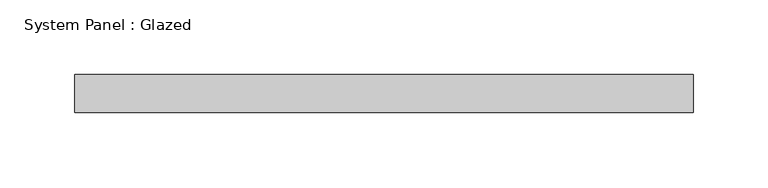
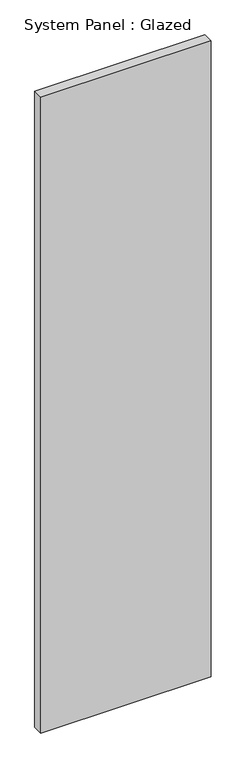
"""IFC4 building model written with IfcOpenShell, lengths in millimetres: plate geometry, System Panel : Glazed."""

from ifc_helpers import new_model, si_unit, origin, origin_with_axes, place, context, project, spatial, polyline, outline, extrude, source, transform, mapped, element, save


def system_panel_glazed_76585487(model_context):
    return source(origin(), model_context, "Body", "SweptSolid", [
        extrude(outline(polyline([(206.375, 19.05), (-206.375, 19.05), (-206.375, 44.45), (206.375, 44.45), (206.375, 19.05)])), origin_with_axes(), (0.0, 0.0, 1.0), 1630.093674),
    ])


if __name__ == "__main__":
    model = new_model("IFC4")
    model_context = context("Model", 3, world=origin())
    ifc_project = project(units=[si_unit("LENGTHUNIT", "METRE", prefix="MILLI")], contexts=[model_context])
    site = spatial("IfcSite", under=ifc_project)
    building = spatial("IfcBuilding", under=site)
    placement = place(None, origin())
    system_panel_glazed_shape = system_panel_glazed_76585487(model_context)
    element("IfcPlate", 1, ObjectType="System Panel : Glazed", at=placement, inside=building, context=model_context, shape_type="MappedRepresentation", body=[
        mapped(system_panel_glazed_shape, transform((0.0, 0.0, 0.0), x_axis=(1.0, 0.0, 0.0), y_axis=(0.0, 1.0, 0.0), z_axis=(0.0, 0.0, 1.0))),
    ])
    save(model, "model.ifc")

# Revit data of these elements
# Type "System Panel : Glazed"
#   Construction Type Id = "GSP4R"
#   Analytic Construction = "1/8 in Pilkington single glazing"
#   Visual Light Transmittance = 0.9
#   Solar Heat Gain Coefficient = 0.86
#   Heat Transfer Coefficient (U) = 1.18115 BTU/(h·ft²·°F)
#   Define Thermal Properties by = 1
# Element 1 (IfcPlate, "System Panel : Glazed")
#   Materials on its faces: "Glass"
# Materials
#   "Glass": class "Glass", colour RGB 0 128 192, transparency 0.75, Description = "Soda Lime Glass", Cost = 0
